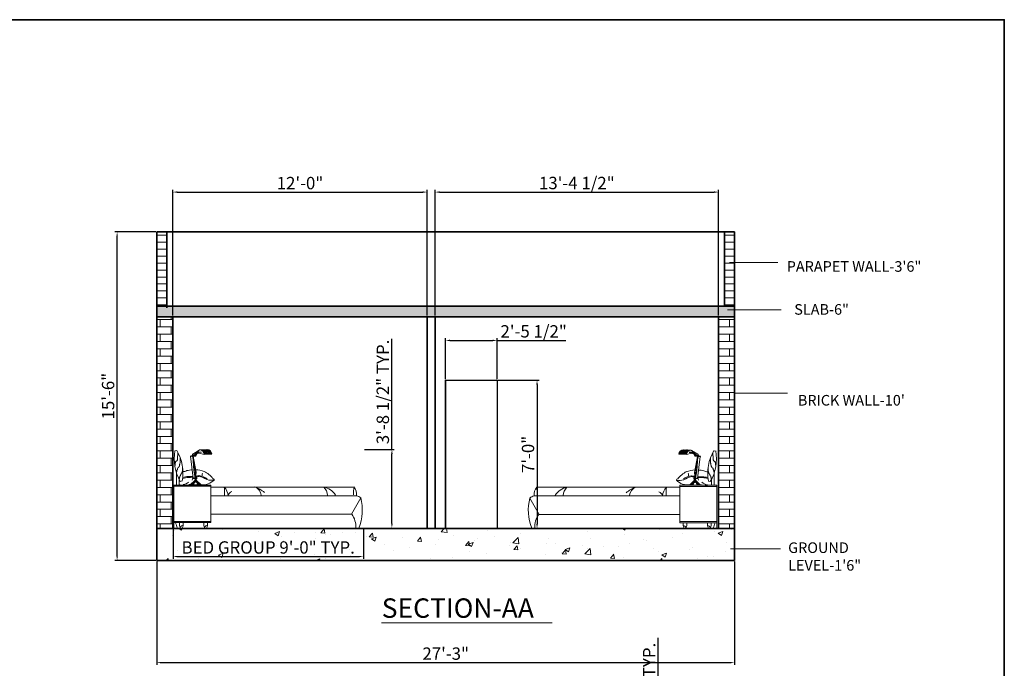
# Model space of a CAD drawing. Units: inches. Extents: x 1863 to 2938, y 1238 to 2492.
# Tile 12 of 12: x 2381 to 2938, y 2125 to 2492. Entities that reach past the tile are written whole.
import ezdxf

# ---------------------------------------------------------------- set-up
doc = ezdxf.new("R2010")
doc.units = ezdxf.units.IN
for name, color, linetype, lineweight in [('A-ANNO-DIMS', 2, 'Continuous', 18), ('A-ANNO-TEXT', 7, 'Continuous', 18), ('A-ANNO-TTLB', 7, 'Continuous', 35), ('A-DOOR', 3, 'Continuous', 25), ('A-FURN', 8, 'Continuous', 18), ('A-SECT', 7, 'Continuous', 35), ('A-SECT-PATT', 8, 'Continuous', 13), ('A-WALL-PATT', 8, 'Continuous', 13)]:
    doc.layers.add(name, color=color, linetype=linetype, lineweight=lineweight)
doc.styles.get("Standard").update_dxf_attribs({"font": 'arial.ttf'})
doc.dimstyles.new('ISO-25', dxfattribs={"dimtxt": 7, "dimasz": 2.5, "dimexe": 1.25, "dimexo": 0.625, "dimtad": 1, "dimdec": 0, "dimlunit": 3, "dimtxsty": 'Standard', "dimcen": 2.5, "dimadec": 0, "dimazin": 0, "dimtfac": 1, "dimtdec": 0, "dimtmove": 0, "dimatfit": 3, "dimfxl": 1, "dimarcsym": 0})

# ---------------------------------------------------------------- blocks, each defined once
blk = doc.blocks.new('A$C244A68C2')
for p, q in [((12, 836), (32, 839)), ((38, 746), (39, 750)), ((38, 739), (38, 746)), ((39, 750), (40, 756)), ((40, 759), (41, 762)), ((40, 756), (40, 759)), ((41, 782), (42, 783)), ((41, 779), (41, 782)), ((41, 775), (41, 779)), ((41, 762), (41, 775)), ((42, 786), (43, 787)), ((42, 783), (42, 786)), ((43, 790), (44, 791)), ((43, 787), (43, 790)), ((44, 791), (44, 812)), ((44, 812), (45, 812)), ((45, 812), (45, 814)), ((67, 766), (67, 705)), ((180, 780), (179, 780)), ((179, 778), (208, 538)), ((179, 778), (180, 777)), ((180, 779), (195, 781)), ((180, 779), (195, 780)), ((180, 778), (195, 777)), ((180, 778), (195, 778)), ((180, 778), (195, 777)), ((180, 777), (208, 539)), ((211, 788), (198, 785)), ((199, 781), (202, 778)), ((201, 778), (199, 781)), ((199, 781), (199, 781)), ((202, 778), (201, 778)), ((201, 774), (209, 776)), ((203, 799), (202, 786)), ((203, 799), (202, 786)), ((205, 801), (203, 801)), ((203, 799), (203, 786)), ((203, 799), (204, 799)), ((204, 799), (205, 787)), ((204, 799), (206, 787)), ((205, 800), (273, 843)), ((205, 801), (275, 843)), ((205, 775), (221, 621)), ((205, 775), (218, 623)), ((208, 782), (260, 825)), ((208, 779), (259, 822)), ((208, 778), (259, 821)), ((239, 779), (208, 779)), ((209, 777), (240, 605)), ((209, 776), (236, 608)), ((214, 783), (238, 783)), ((234, 779), (259, 822)), ((239, 779), (259, 822)), ((299, 822), (259, 822)), ((299, 821), (259, 821)), ((260, 814), (259, 814)), ((264, 816), (268, 815)), ((268, 815), (264, 816)), ((264, 816), (264, 816)), ((268, 815), (268, 815)), ((268, 810), (273, 811)), ((328, 797), (273, 811)), ((278, 845), (361, 850)), ((410, 801), (328, 797)), ((11, 670), (12, 676)), ((11, 670), (11, 670)), ((12, 676), (13, 681)), ((13, 681), (15, 686)), ((15, 695), (16, 699)), ((15, 686), (15, 695)), ((16, 707), (17, 708)), ((16, 699), (16, 707)), ((17, 712), (18, 715)), ((17, 708), (17, 712)), ((18, 716), (19, 719)), ((18, 715), (18, 716)), ((19, 719), (20, 719)), ((20, 719), (23, 722)), ((23, 722), (27, 723)), ((27, 724), (30, 725)), ((27, 723), (27, 724)), ((30, 725), (31, 728)), ((31, 728), (32, 729)), ((32, 729), (36, 732)), ((36, 732), (37, 735)), ((37, 736), (38, 739)), ((37, 735), (37, 736)), ((40, 640), (39, 637)), ((41, 644), (40, 640)), ((42, 650), (41, 646)), ((41, 646), (41, 645)), ((41, 645), (41, 644)), ((43, 651), (42, 650)), ((44, 652), (43, 652)), ((43, 652), (43, 651)), ((45, 652), (44, 652)), ((46, 653), (45, 652)), ((47, 654), (46, 653)), ((48, 655), (47, 654)), ((49, 655), (48, 655)), ((50, 656), (49, 655)), ((51, 657), (50, 656)), ((52, 657), (51, 657)), ((53, 658), (52, 658)), ((52, 658), (52, 657)), ((54, 659), (53, 658)), ((55, 662), (54, 659)), ((57, 663), (55, 662)), ((58, 665), (57, 665)), ((57, 665), (57, 663)), ((59, 667), (58, 666)), ((58, 666), (58, 665)), ((60, 671), (59, 668)), ((59, 668), (59, 667)), ((61, 675), (60, 672)), ((60, 672), (60, 671)), ((62, 679), (61, 676)), ((61, 676), (61, 675)), ((63, 683), (62, 682)), ((62, 682), (62, 679)), ((64, 692), (63, 688)), ((63, 688), (63, 683)), ((66, 699), (64, 692)), ((67, 705), (66, 699)), ((92, 616), (92, 640)), ((92, 640), (93, 640)), ((93, 640), (93, 659)), ((27, 602), (27, 465)), ((30, 603), (29, 602)), ((29, 602), (29, 598)), ((29, 598), (29, 598)), ((31, 611), (30, 610)), ((30, 610), (30, 603)), ((32, 614), (31, 613)), ((31, 613), (31, 611)), ((33, 619), (32, 618)), ((32, 618), (32, 614)), ((34, 624), (33, 620)), ((33, 620), (33, 619)), ((35, 627), (34, 626)), ((34, 626), (34, 624)), ((36, 628), (35, 627)), ((37, 631), (36, 630)), ((36, 630), (36, 628)), ((38, 634), (37, 631)), ((39, 637), (38, 636)), ((38, 636), (38, 634)), ((59, 526), (59, 536)), ((59, 536), (60, 536)), ((60, 536), (60, 543)), ((60, 543), (61, 543)), ((61, 543), (61, 544)), ((61, 544), (62, 544)), ((62, 544), (62, 549)), ((62, 549), (63, 549)), ((63, 549), (63, 552)), ((63, 552), (64, 552)), ((64, 552), (64, 556)), ((64, 556), (65, 556)), ((65, 559), (65, 561)), ((65, 561), (66, 561)), ((65, 556), (65, 559)), ((65, 559), (65, 559)), ((66, 561), (66, 562)), ((66, 562), (67, 562)), ((67, 562), (67, 564)), ((67, 564), (68, 564)), ((68, 564), (69, 564)), ((69, 565), (70, 566)), ((69, 564), (69, 565)), ((70, 566), (71, 567)), ((71, 567), (72, 571)), ((72, 572), (73, 573)), ((72, 571), (72, 572)), ((73, 574), (74, 575)), ((73, 573), (73, 574)), ((74, 575), (74, 577)), ((74, 577), (75, 577)), ((75, 579), (76, 580)), ((75, 577), (75, 579)), ((76, 580), (76, 582)), ((76, 582), (77, 582)), ((77, 583), (78, 584)), ((77, 582), (77, 583)), ((78, 588), (79, 589)), ((78, 587), (78, 588)), ((78, 586), (78, 587)), ((78, 584), (78, 586)), ((79, 589), (80, 589)), ((80, 589), (81, 590)), ((81, 590), (82, 591)), ((82, 591), (83, 591)), ((83, 591), (83, 592)), ((83, 592), (84, 592)), ((84, 592), (85, 593)), ((85, 594), (86, 595)), ((85, 593), (85, 594)), ((86, 595), (87, 599)), ((87, 599), (88, 600)), ((88, 600), (88, 604)), ((88, 604), (89, 604)), ((89, 604), (89, 606)), ((89, 606), (90, 606)), ((90, 606), (90, 608)), ((90, 608), (91, 608)), ((91, 612), (92, 613)), ((91, 608), (91, 612)), ((92, 615), (92, 616)), ((92, 613), (92, 615)), ((210, 539), (208, 539)), ((209, 538), (209, 538)), ((209, 537), (227, 536)), ((209, 537), (227, 536)), ((209, 537), (210, 537)), ((210, 538), (228, 540)), ((210, 538), (228, 540)), ((210, 537), (227, 537)), ((218, 623), (230, 541)), ((221, 621), (230, 541)), ((230, 536), (234, 535)), ((233, 534), (230, 536)), ((230, 536), (230, 536)), ((245, 544), (231, 542)), ((234, 535), (233, 534)), ((236, 608), (234, 542)), ((240, 605), (234, 543)), ((234, 564), (237, 564)), ((234, 564), (238, 564)), ((237, 564), (234, 564)), ((234, 561), (238, 562)), ((234, 561), (237, 562)), ((235, 561), (234, 542)), ((235, 563), (238, 564)), ((236, 561), (235, 542)), ((235, 561), (235, 542)), ((237, 561), (238, 543)), ((237, 561), (238, 543)), ((0, 0), (0, 465)), ((0, 465), (400, 465)), ((0, 453), (400, 453)), ((57, 529), (57, 465)), ((90, 509), (70, 505)), ((232, 519), (176, 467)), ((176, 467), (296, 467)), ((176, 466), (176, 465)), ((176, 465), (297, 465)), ((232, 519), (232, 529)), ((232, 519), (242, 519)), ((233, 529), (247, 532)), ((233, 519), (233, 530)), ((233, 519), (233, 529)), ((234, 519), (234, 530)), ((236, 519), (236, 530)), ((241, 519), (241, 531)), ((242, 519), (242, 531)), ((242, 519), (242, 531)), ((296, 467), (242, 519)), ((297, 465), (297, 466)), ((400, 465), (400, 60)), ((400, 444), (1950, 444)), ((400, 349), (1978, 349)), ((2023, 327), (1924, 150)), ((1924, 150), (400, 150)), ((400, 72), (0, 72)), ((400, 60), (0, 60)), ((2000, 0), (0, 0)), ((69, 0), (39, 0)), ((1970, 0), (2000, 0))]:
    blk.add_line(p, q)
for centre in [(200, 780), (266, 815)]:
    blk.add_circle(centre, 5.65)
for centre, radius, start, end in [((490, 750), 486, 169.7597, 210.2403), ((-388, 595), 486, 349.7597, 30.2403), ((179, 778), 1.33, 113.0446, 219.3657), ((179, 778), 0.665, 242.9995, 272.6955), ((179, 779), 0.499, 23.7236, 96.4275), ((178, 779), 1.65, 302.8629, 16.2974), ((178, 779), 0.993, 300.7534, 34.996), ((179, 779), 1.41, 300.6413, 40.8102), ((204, 800), 1.41, 113.0446, 219.3657), ((202, 800), 1.74, 302.8629, 16.2974), ((203, 800), 0.527, 23.7236, 96.4275), ((202, 800), 1.05, 300.7534, 34.996), ((203, 799), 0.701, 242.9995, 272.6955), ((203, 800), 1.49, 302.2124, 40.8102), ((212, 780), 4.54, 146.492, 201.5266), ((206, 786), 10.1, 287.8935, 311.557), ((208, 782), 6.25, 5.1761, 68.5727), ((222, 781), 2.75, 324.8716, 43.8406), ((223, 781), 2.75, 324.8716, 43.8406), ((289, 817), 30.1, 110.5321, 185.4329), ((278, 795), 50.1, 2.0446, 89.1762), ((285, 795), 50.1, 2.62, 89.1762), ((292, 797), 50.1, 0.9228, 81.157), ((309, 797), 50.1, 2.0096, 97.716), ((300, 797), 50.1, 1.4059, 83.743), ((317, 797), 50.1, 2.0154, 97.6411), ((326, 798), 50.1, 2.0212, 97.5649), ((335, 798), 50.1, 2.0446, 89.8396), ((344, 798), 50.1, 2.6306, 89.1762), ((352, 800), 50.1, 1.5315, 84.5393), ((360, 800), 50.1, 2.0446, 89.1762), ((188, 153), 396, 94.4237, 103.6768), ((188, 153), 406, 94.4237, 103.1785), ((102, 690), 79.6, 266.5082, 300.0492), ((220, 319), 312, 94.2751, 104.4301), ((161, 1136), 579, 269.5712, 274.3558), ((161, 1136), 588, 269.5712, 274.3996), ((247, 517), 49.6, 143.8256, 177.3514), ((208, 538), 0.549, 47.8474, 120.5513), ((209, 538), 1.47, 137.1685, 243.4896), ((208, 538), 1.09, 324.8773, 59.1199), ((207, 538), 1.82, 326.9868, 40.4213), ((209, 537), 0.731, 267.1233, 296.8194), ((209, 538), 1.46, 324.571, 61.0928), ((225, 543), 7.93, 47.5431, 107.8683), ((225, 542), 8.22, 45.6214, 105.6239), ((233, 536), 6.38, 116.914, 258.5276), ((233, 535), 5.43, 117.012, 254.6625), ((231, 538), 3.62, 54.3229, 113.5884), ((231, 537), 3.42, 88.4984, 107.6275), ((228, 535), 5.38, 317.0855, 61.4366), ((234, 562), 1.61, 113.0446, 254.6581), ((234, 563), 0.913, 50.4535, 109.7189), ((234, 563), 0.864, 84.629, 103.758), ((234, 562), 1.37, 113.1426, 250.793), ((233, 562), 1.64, 295.9717, 55.8772), ((233, 562), 1.1, 315.8031, 60.4731), ((234, 562), 0.947, 260.6456, 290.3416), ((230, 535), 6.5, 299.8411, 59.7467), ((220, 319), 312, 69.9385, 87.115), ((237, 563), 1.64, 301.136, 71.7859), ((161, 1136), 579, 277.6123, 280.9344), ((161, 1136), 588, 277.4426, 280.9344), ((243, 538), 6.48, 305.0055, 75.6553), ((224, 315), 248, 57.6744, 78.9535), ((224, 315), 258, 57.6744, 78.9535), ((336, 576), 31.1, 141.8486, 203.2325), ((219, 384), 253, 36.2927, 64.7019), ((422, 521), 13.7, 351.6123, 92.6357), ((116, 662), 200, 252.6794, 279.5672), ((84, 593), 124, 277.542, 309.9334), ((258, 63), 417, 100.9046, 105.0614), ((176, 466), 0.81, 90, 180), ((232, 533), 3.75, 264.5151, 294.2111), ((311, 645), 177, 264.2572, 314.636), ((296, 466), 0.81, 360, 90), ((405, 650), 134, 250.0666, 283.0972), ((-655, 373), 1203, 358.8801, 3.375), ((439, 340), 148, 3.5443, 44.2346), ((834, 341), 112, 7.9131, 67.3602), ((739, 84), 386, 51.1586, 69.1463), ((1526, 348), 136, 1.9043, 44.8247), ((1591, 263), 183, 30.3408, 80.0939), ((2269, 374), 326, 167.6533, 182.7628), ((1855, 364), 124, 353.2313, 40.2408), ((648, 336), 61.5, 109.2631, 167.6798), ((1967, 270), 80, 45, 81.6372), ((1523, 198), 517, 337.4954, 14.4201), ((1736, 10), 235, 357.5091, 36.5889), ((514, 197), 514, 195.5801, 202.5597), ((158, 45), 98.5, 171.4719, 207.4528), ((107, -17), 46.6, 97.2386, 147.0434), ((301, 10), 232, 181.8198, 182.4988), ((4, 45), 98.5, 332.5472, 8.5281), ((422, 45), 98.5, 171.4719, 207.4528), ((370, -17), 46.6, 97.2386, 147.0434), ((267, 45), 98.5, 332.5472, 8.5281)]:
    blk.add_arc(centre, radius, start, end)
for points in [[(200, 774), (201, 774), (201, 775), (202, 775), (202, 775), (203, 776), (203, 777), (204, 778), (204, 779), (204, 781), (204, 781), (203, 782), (203, 783), (202, 784), (202, 784), (201, 784), (201, 784), (200, 784), (200, 784), (200, 784), (200, 784)], [(266, 810), (267, 810), (267, 810), (268, 811), (268, 811), (269, 812), (269, 813), (270, 814), (270, 815), (270, 817), (269, 817), (269, 818), (268, 819), (268, 820), (267, 820), (266, 820), (266, 820), (266, 820), (266, 820), (266, 820), (266, 820)], [(231, 530), (232, 530), (232, 530), (233, 531), (234, 531), (234, 532), (235, 533), (235, 534), (235, 535), (235, 537), (235, 537), (234, 538), (234, 539), (233, 540), (233, 540), (232, 540), (232, 540), (231, 540), (231, 540), (231, 540), (231, 540)], [(234, 561), (234, 561), (234, 561), (234, 561), (234, 561), (234, 562), (234, 562), (235, 562), (235, 562), (235, 563), (235, 563), (234, 563), (234, 563), (234, 563), (234, 564), (234, 564), (234, 564), (234, 564), (234, 564), (234, 564), (234, 564)]]:
    blk.add_open_spline(points, degree=3, knots=[3.294068, 3.294068, 3.294068, 3.294068, 3.647859, 3.647859, 4.043866, 4.043866, 4.439873, 4.439873, 4.83588, 4.83588, 5.231886, 5.231886, 5.627893, 5.627893, 6.0239, 6.0239, 6.283185, 6.283185, 6.283185, 6.295262, 6.295262, 6.295262, 6.295262])
for p in [(202, 786), (202, 785), (203, 786), (203, 785), (204, 786), (204, 786), (204, 785), (204, 784), (205, 786), (205, 786), (205, 785), (205, 784), (205, 783), (205, 776), (205, 775), (205, 775), (205, 775), (206, 786), (206, 786), (206, 785), (206, 777), (206, 776), (206, 776), (206, 776), (207, 786), (207, 783), (208, 787), (208, 786), (208, 786), (208, 785), (208, 777), (208, 777), (208, 777), (209, 787), (209, 787), (209, 787), (209, 786), (209, 785), (209, 784), (209, 784), (209, 777), (209, 777), (210, 787), (210, 787), (210, 787), (210, 787), (210, 786), (210, 778), (210, 777), (211, 787), (211, 786), (211, 778), (211, 777), (212, 787), (212, 786), (212, 786), (212, 784), (213, 785), (234, 542), (234, 541), (234, 541), (235, 542), (235, 541), (235, 541), (235, 540), (236, 542), (236, 541), (236, 541), (236, 541), (236, 540), (236, 540), (237, 543), (237, 542), (237, 542), (237, 541), (237, 541), (237, 541), (237, 540), (238, 543), (238, 542), (238, 542), (238, 542), (238, 540), (238, 538), (239, 542), (239, 541), (239, 541), (239, 539), (240, 543), (240, 541), (240, 541), (241, 543), (241, 543), (241, 542), (242, 543), (242, 543), (242, 542), (242, 542), (242, 540), (243, 543), (243, 543), (243, 543), (244, 544), (244, 543), (244, 542), (244, 540), (244, 540), (245, 544), (245, 544), (245, 544), (245, 543), (245, 533), (245, 533), (245, 533), (246, 543), (246, 543), (246, 542), (246, 534), (246, 533), (247, 543), (247, 543), (247, 541), (247, 535), (247, 534), (247, 534), (248, 541), (248, 537), (248, 536), (248, 535), (248, 535), (248, 535), (248, 535), (248, 534), (181, 468), (182, 469), (183, 470), (185, 472), (185, 471), (186, 470), (186, 470), (186, 468), (186, 468), (186, 467), (187, 473), (188, 474), (188, 473), (188, 471), (188, 471), (188, 470), (189, 473), (190, 474), (190, 474), (190, 470), (190, 470), (191, 478), (191, 474), (191, 471), (193, 474), (193, 474), (193, 473), (193, 469), (194, 478), (194, 473), (194, 471), (195, 476), (195, 473), (195, 471), (196, 477), (197, 480), (197, 473), (197, 469), (198, 470), (198, 469), (198, 469), (199, 482), (201, 482), (201, 470), (202, 486), (202, 482), (202, 469), (204, 484), (205, 481), (206, 485), (206, 477), (206, 469), (206, 468), (207, 491), (207, 489), (207, 487), (207, 474), (207, 473), (208, 487), (208, 482), (209, 491), (210, 491), (210, 489), (210, 484), (210, 472), (211, 496), (211, 470), (211, 470), (212, 493), (212, 485), (212, 475), (214, 498), (214, 487), (215, 500), (215, 499), (215, 476), (216, 500), (216, 498), (216, 497), (216, 489), (216, 489), (216, 484), (216, 480), (217, 502), (217, 499), (218, 504), (219, 504), (219, 503), (219, 502), (219, 501), (219, 483), (220, 506), (220, 505), (221, 504), (221, 504), (221, 498), (221, 492), (222, 506), (222, 506), (222, 494), (223, 508), (223, 501), (223, 498), (224, 508), (224, 506), (224, 506), (224, 504), (225, 510), (225, 508), (225, 498), (226, 511), (226, 509), (226, 503), (227, 513), (227, 511), (227, 507), (227, 504), (228, 514), (228, 511), (228, 508), (229, 512), (229, 512), (229, 511), (229, 508), (229, 507), (230, 513), (230, 512), (230, 511), (230, 503), (231, 516), (231, 515), (231, 514), (231, 507), (232, 516), (233, 517), (233, 514), (233, 512), (233, 510), (234, 517), (234, 513), (234, 512), (235, 519), (235, 517), (235, 517), (235, 516), (235, 515), (235, 514), (235, 512), (236, 532), (236, 517), (236, 517), (236, 497), (237, 532), (237, 532), (237, 504), (237, 500), (238, 532), (238, 515), (238, 512), (238, 497), (239, 532), (239, 532), (239, 508), (240, 532), (241, 533), (241, 533), (243, 533), (243, 532), (243, 513), (243, 512), (243, 506), (244, 514), (244, 512), (244, 511), (244, 508), (245, 513), (245, 511), (245, 511), (246, 511), (246, 506), (246, 502), (246, 500), (247, 510), (247, 509), (248, 508), (248, 495), (249, 508), (249, 506), (249, 506), (249, 504), (249, 502), (250, 508), (250, 506), (251, 506), (251, 504), (251, 498), (251, 492), (252, 506), (252, 505), (252, 504), (253, 467), (254, 504), (254, 503), (254, 502), (254, 501), (254, 483), (254, 473), (255, 504), (255, 499), (255, 495), (255, 493), (255, 486), (255, 484), (256, 502), (256, 500), (256, 498), (256, 497), (257, 500), (257, 499), (258, 498), (258, 487), (258, 478), (258, 471), (259, 498), (259, 495), (259, 491), (260, 494), (260, 493), (260, 490), (260, 479), (260, 472), (260, 467), (261, 496), (261, 489), (261, 485), (262, 488), (262, 487), (262, 484), (263, 491), (263, 489), (263, 484), (264, 491), (264, 481), (264, 471), (264, 471), (265, 491), (265, 489), (265, 487), (265, 487), (265, 482), (266, 485), (266, 484), (266, 470), (266, 467), (267, 478), (267, 469), (267, 469), (267, 467), (268, 481), (269, 484), (269, 482), (269, 481), (269, 473), (270, 486), (270, 482), (270, 477), (270, 469), (271, 488), (271, 482), (271, 470), (273, 476), (273, 470), (274, 482), (274, 469), (276, 480), (277, 480), (280, 471), (280, 469), (281, 474), (281, 471), (282, 475), (282, 470), (284, 471), (285, 473), (285, 470), (287, 470), (288, 470), (288, 469), (290, 469), (291, 467)]:
    blk.add_point(p)
blk = doc.blocks.new('*D38')
at = {"layer": 'A-ANNO-DIMS', "color": 0, "lineweight": -2, "transparency": 16777216}
for p, q in [((2467.74, 2203.68), (2467.74, 2186.89)), ((2575.51, 2203.68), (2575.51, 2186.89)), ((2470.24, 2188.14), (2573.01, 2188.14))]:
    blk.add_line(p, q, dxfattribs=at)
at = {"layer": 'A-ANNO-DIMS', "color": 0, "transparency": 16777216}
for points in [[(2470.24, 2188.55), (2470.24, 2187.72), (2467.74, 2188.14)], [(2573.01, 2188.55), (2573.01, 2187.72), (2575.51, 2188.14)]]:
    blk.add_solid(points, dxfattribs=at)
at = {"layer": 'Defpoints', "color": 0, "transparency": 16777216}
for p in [(2467.74, 2204.3), (2575.51, 2204.3), (2575.51, 2188.14)]:
    blk.add_point(p, dxfattribs=at)
at = {"layer": 'A-ANNO-DIMS', "color": 0, "transparency": 16777216, "insert": (2521.62, 2192.38), "char_height": 7, "attachment_point": 5}
blk.add_mtext('BED GROUP 9\'-0" TYP.', dxfattribs=at)
blk = doc.blocks.new('*D39')
at = {"layer": 'A-ANNO-DIMS', "color": 0, "lineweight": -2, "transparency": 16777216}
for p, q in [((2591.67, 2248.76), (2591.67, 2311.48)), ((2576.13, 2248.76), (2592.92, 2248.76)), ((2591.67, 2206.8), (2591.67, 2246.26)), ((2576.13, 2204.3), (2592.92, 2204.3))]:
    blk.add_line(p, q, dxfattribs=at)
at = {"layer": 'A-ANNO-DIMS', "color": 0, "transparency": 16777216}
for points in [[(2591.26, 2246.26), (2592.09, 2246.26), (2591.67, 2248.76)], [(2591.26, 2206.8), (2592.09, 2206.8), (2591.67, 2204.3)]]:
    blk.add_solid(points, dxfattribs=at)
at = {"layer": 'Defpoints', "color": 0, "transparency": 16777216}
for p in [(2575.51, 2248.76), (2591.67, 2248.76), (2575.51, 2204.3)]:
    blk.add_point(p, dxfattribs=at)
at = {"layer": 'A-ANNO-DIMS', "color": 0, "transparency": 16777216, "insert": (2587.43, 2281.37), "char_height": 7, "attachment_point": 5, "rotation": 90}
blk.add_mtext('3\'-8 1/2" TYP.', dxfattribs=at)
blk = doc.blocks.new('*D44')
at = {"layer": 'A-ANNO-DIMS', "color": 0, "lineweight": -2, "transparency": 16777216}
for p, q in [((2742.49, 2018.92), (2742.49, 2142.19)), ((2739.01, 2018.92), (2743.74, 2018.92)), ((2742.49, 1994.04), (2742.49, 2016.42)), ((2739.01, 1991.54), (2743.74, 1991.54))]:
    blk.add_line(p, q, dxfattribs=at)
at = {"layer": 'A-ANNO-DIMS', "color": 0, "transparency": 16777216}
for points in [[(2742.07, 2016.42), (2742.91, 2016.42), (2742.49, 2018.92)], [(2742.07, 1994.04), (2742.91, 1994.04), (2742.49, 1991.54)]]:
    blk.add_solid(points, dxfattribs=at)
at = {"layer": 'Defpoints', "color": 0, "transparency": 16777216}
for p in [(2738.38, 2018.92), (2742.49, 2018.92), (2738.38, 1991.54)]:
    blk.add_point(p, dxfattribs=at)
at = {"layer": 'A-ANNO-DIMS', "color": 0, "transparency": 16777216, "insert": (2738.24, 2081.8), "char_height": 7, "attachment_point": 5, "rotation": 90}
blk.add_mtext('BATH DOOR 2\'-3 1/2" TYP.', dxfattribs=at)
blk = doc.blocks.new('*D87')
at = {"layer": 'A-ANNO-DIMS', "color": 0, "lineweight": -2, "transparency": 16777216}
for p, q in [((2458.63, 2185.37), (2458.63, 2126.81)), ((2785.63, 2185.37), (2785.63, 2126.81)), ((2461.13, 2128.06), (2783.13, 2128.06))]:
    blk.add_line(p, q, dxfattribs=at)
at = {"layer": 'A-ANNO-DIMS', "color": 0, "transparency": 16777216}
for points in [[(2461.13, 2128.47), (2461.13, 2127.64), (2458.63, 2128.06)], [(2783.13, 2128.47), (2783.13, 2127.64), (2785.63, 2128.06)]]:
    blk.add_solid(points, dxfattribs=at)
at = {"layer": 'Defpoints', "color": 0, "transparency": 16777216}
for p in [(2458.63, 2185.99), (2785.63, 2185.99), (2785.63, 2128.06)]:
    blk.add_point(p, dxfattribs=at)
at = {"layer": 'A-ANNO-DIMS', "color": 0, "transparency": 16777216, "insert": (2622.13, 2132.26), "char_height": 7, "attachment_point": 5}
blk.add_mtext('27\'-3"', dxfattribs=at)
blk = doc.blocks.new('*D88')
at = {"layer": 'A-ANNO-DIMS', "color": 0, "lineweight": -2, "transparency": 16777216}
for p, q in [((2458.01, 2371.99), (2434.83, 2371.99)), ((2436.08, 2188.49), (2436.08, 2369.49)), ((2458.01, 2185.99), (2434.83, 2185.99))]:
    blk.add_line(p, q, dxfattribs=at)
at = {"layer": 'A-ANNO-DIMS', "color": 0, "transparency": 16777216}
for points in [[(2435.66, 2369.49), (2436.5, 2369.49), (2436.08, 2371.99)], [(2435.66, 2188.49), (2436.5, 2188.49), (2436.08, 2185.99)]]:
    blk.add_solid(points, dxfattribs=at)
at = {"layer": 'Defpoints', "color": 0, "transparency": 16777216}
for p in [(2436.08, 2371.99), (2458.63, 2371.99), (2458.63, 2185.99)]:
    blk.add_point(p, dxfattribs=at)
at = {"layer": 'A-ANNO-DIMS', "color": 0, "transparency": 16777216, "insert": (2431.88, 2278.99), "char_height": 7, "attachment_point": 5, "rotation": 90}
blk.add_mtext('15\'-6"', dxfattribs=at)
blk = doc.blocks.new('*D89')
at = {"layer": 'A-ANNO-DIMS', "color": 0, "lineweight": -2, "transparency": 16777216}
for p, q in [((2467.63, 2324.62), (2467.63, 2395.79)), ((2470.13, 2394.54), (2609.13, 2394.54)), ((2611.63, 2324.62), (2611.63, 2395.79))]:
    blk.add_line(p, q, dxfattribs=at)
at = {"layer": 'A-ANNO-DIMS', "color": 0, "transparency": 16777216}
for points in [[(2470.13, 2394.96), (2470.13, 2394.12), (2467.63, 2394.54)], [(2609.13, 2394.96), (2609.13, 2394.12), (2611.63, 2394.54)]]:
    blk.add_solid(points, dxfattribs=at)
at = {"layer": 'Defpoints', "color": 0, "transparency": 16777216}
for p in [(2611.63, 2394.54), (2467.63, 2323.99), (2611.63, 2323.99)]:
    blk.add_point(p, dxfattribs=at)
at = {"layer": 'A-ANNO-DIMS', "color": 0, "transparency": 16777216, "insert": (2539.63, 2398.74), "char_height": 7, "attachment_point": 5}
blk.add_mtext('12\'-0"', dxfattribs=at)
blk = doc.blocks.new('*D90')
at = {"layer": 'A-ANNO-DIMS', "color": 0, "lineweight": -2, "transparency": 16777216}
for p, q in [((2616.13, 2324.62), (2616.13, 2395.79)), ((2618.63, 2394.54), (2774.13, 2394.54)), ((2776.63, 2324.62), (2776.63, 2395.79))]:
    blk.add_line(p, q, dxfattribs=at)
at = {"layer": 'A-ANNO-DIMS', "color": 0, "transparency": 16777216}
for points in [[(2618.63, 2394.96), (2618.63, 2394.12), (2616.13, 2394.54)], [(2774.13, 2394.96), (2774.13, 2394.12), (2776.63, 2394.54)]]:
    blk.add_solid(points, dxfattribs=at)
at = {"layer": 'Defpoints', "color": 0, "transparency": 16777216}
for p in [(2776.63, 2394.54), (2616.13, 2323.99), (2776.63, 2323.99)]:
    blk.add_point(p, dxfattribs=at)
at = {"layer": 'A-ANNO-DIMS', "color": 0, "transparency": 16777216, "insert": (2696.38, 2398.79), "char_height": 7, "attachment_point": 5}
blk.add_mtext('13\'-4 1/2"', dxfattribs=at)
blk = doc.blocks.new('*D91')
at = {"layer": 'A-ANNO-DIMS', "color": 0, "lineweight": -2, "transparency": 16777216}
for p, q in [((2651.91, 2287.99), (2675.09, 2287.99)), ((2673.84, 2285.49), (2673.84, 2206.49)), ((2651.91, 2203.99), (2675.09, 2203.99))]:
    blk.add_line(p, q, dxfattribs=at)
at = {"layer": 'A-ANNO-DIMS', "color": 0, "transparency": 16777216}
for points in [[(2673.42, 2285.49), (2674.25, 2285.49), (2673.84, 2287.99)], [(2673.42, 2206.49), (2674.25, 2206.49), (2673.84, 2203.99)]]:
    blk.add_solid(points, dxfattribs=at)
at = {"layer": 'Defpoints', "color": 0, "transparency": 16777216}
for p in [(2651.29, 2287.99), (2651.29, 2203.99), (2673.84, 2203.99)]:
    blk.add_point(p, dxfattribs=at)
at = {"layer": 'A-ANNO-DIMS', "color": 0, "transparency": 16777216, "insert": (2669.64, 2245.99), "char_height": 7, "attachment_point": 5, "rotation": 90}
blk.add_mtext('7\'-0"', dxfattribs=at)
blk = doc.blocks.new('*D92')
at = {"layer": 'A-ANNO-DIMS', "color": 0, "lineweight": -2, "transparency": 16777216}
for p, q in [((2622.04, 2288.62), (2622.04, 2311.79)), ((2624.54, 2310.54), (2648.79, 2310.54)), ((2651.29, 2288.62), (2651.29, 2311.79)), ((2651.29, 2310.54), (2690.08, 2310.54))]:
    blk.add_line(p, q, dxfattribs=at)
at = {"layer": 'A-ANNO-DIMS', "color": 0, "transparency": 16777216}
for points in [[(2624.54, 2310.96), (2624.54, 2310.12), (2622.04, 2310.54)], [(2648.79, 2310.96), (2648.79, 2310.12), (2651.29, 2310.54)]]:
    blk.add_solid(points, dxfattribs=at)
at = {"layer": 'Defpoints', "color": 0, "transparency": 16777216}
for p in [(2651.29, 2310.54), (2622.04, 2287.99), (2651.29, 2287.99)]:
    blk.add_point(p, dxfattribs=at)
at = {"layer": 'A-ANNO-DIMS', "color": 0, "transparency": 16777216, "insert": (2671.93, 2314.78), "char_height": 7, "attachment_point": 5}
blk.add_mtext('2\'-5 1/2"', dxfattribs=at)

msp = doc.modelspace()

# ---------------------------------------------------------------- hatches: boundary and pattern name
at = {"layer": 'A-SECT-PATT'}
h = msp.add_hatch(dxfattribs=at)
h.set_pattern_fill('AR-CONC', color=256, scale=0.045, style=0)
h.paths.add_polyline_path([(2458.63, 2323.99), (2785.63, 2323.99), (2785.63, 2329.99), (2458.63, 2329.99)])
h = msp.add_hatch(dxfattribs=at)
h.set_pattern_fill('AR-CONC', color=256, scale=0.15, style=0)
h.paths.add_polyline_path([(2458.63, 2185.99), (2785.63, 2185.99), (2785.63, 2203.99), (2458.63, 2203.99)])
at = {"layer": 'A-WALL-PATT'}
h = msp.add_hatch(dxfattribs=at)
h.set_pattern_fill('LINE', color=256, scale=1.24, style=0)
h.paths.add_polyline_path([(2458.63, 2329.99), (2464.19, 2329.99), (2464.19, 2371.99), (2458.63, 2371.99)])
h = msp.add_hatch(dxfattribs=at)
h.set_pattern_fill('LINE', color=256, scale=1.24, style=0)
h.paths.add_polyline_path([(2780.05, 2329.99), (2785.63, 2329.99), (2785.63, 2371.99), (2780.05, 2371.99)])
h = msp.add_hatch(dxfattribs=at)
h.set_pattern_fill('AR-BRSTD', color=256, scale=0.061, style=0)
h.paths.add_polyline_path([(2458.63, 2203.99), (2467.63, 2203.99), (2467.63, 2323.99), (2458.63, 2323.99)])
h = msp.add_hatch(dxfattribs=at)
h.set_pattern_fill('AR-BRSTD', color=256, scale=0.061, style=0)
h.paths.add_polyline_path([(2776.63, 2203.99), (2785.63, 2203.99), (2785.63, 2323.99), (2776.63, 2323.99)])

# ---------------------------------------------------------------- linework, layer by layer
at = {"layer": 'A-ANNO-TEXT'}
for p, q in [((2782.84, 2354.68), (2810.09, 2354.68)), ((2781.77, 2327.92), (2811.99, 2327.92)), ((2785.63, 2280.67), (2815.7, 2280.67)), ((2783.39, 2192.59), (2811.67, 2192.59)), ((2585.71, 2150.61), (2682.44, 2150.61))]:
    msp.add_line(p, q, dxfattribs=at)
at = {"layer": 'A-ANNO-TTLB'}
msp.add_lwpolyline([(1863.2, 2492.19), (2938.41, 2492.19), (2938.41, 1253.47), (1863.2, 1253.47)], close=True, dxfattribs=at)
at = {"layer": 'A-DOOR'}
for p, q in [((2622.04, 2287.99), (2622.04, 2203.99)), ((2622.04, 2203.99), (2622.04, 2287.99)), ((2622.04, 2287.99), (2651.29, 2287.99)), ((2651.29, 2287.99), (2651.29, 2203.99))]:
    msp.add_line(p, q, dxfattribs=at)
at = {"layer": 'A-SECT'}
for p, q in [((2458.63, 2371.99), (2458.63, 2185.99)), ((2458.63, 2371.99), (2785.63, 2371.99)), ((2464.19, 2329.05), (2464.19, 2371.99)), ((2780.05, 2329.99), (2780.05, 2371.99)), ((2785.63, 2371.99), (2785.63, 2185.99)), ((2458.63, 2329.99), (2785.63, 2329.99)), ((2458.63, 2323.99), (2785.63, 2323.99)), ((2467.63, 2323.99), (2467.63, 2203.99)), ((2611.63, 2323.99), (2611.63, 2203.99)), ((2616.13, 2323.99), (2616.13, 2203.99)), ((2776.63, 2323.99), (2776.63, 2203.99)), ((2458.63, 2203.99), (2785.63, 2203.99)), ((2458.63, 2185.99), (2785.63, 2185.99))]:
    msp.add_line(p, q, dxfattribs=at)

# ---------------------------------------------------------------- block references
at = {"layer": 'A-FURN', "yscale": 0.0523142138983917, "zscale": 0.0523142138983917}
for p, xscale in [((2468.2, 2204.3), 0.0523142138983917), ((2775.63, 2204.18), -0.0523142138983917)]:
    msp.add_blockref('A$C244A68C2', p, dxfattribs=dict(at, xscale=xscale))

# ---------------------------------------------------------------- texts
at = {"layer": 'A-ANNO-TEXT', "attachment_point": 1}
for s, width, insert, char_height in [('PARAPET WALL-3\'6"', 114.3843, (2815.22, 2355.43), 6), ('SLAB-6"', 81.9754, (2819.48, 2331.1), 6), ("BRICK WALL-10'", 211.4644, (2821.53, 2279.64), 6), ('GROUND LEVEL-1\'6"', 65.94, (2816.02, 2196.17), 6), ('SECTION-AA', 293.6592, (2585.9, 2164.45), 11)]:
    msp.add_mtext_dynamic_manual_height_columns(s, width=width, gutter_width=12.5, heights=[0], dxfattribs=dict(at, insert=insert, char_height=char_height))

# ---------------------------------------------------------------- dimensions: what is measured, and where the dimension line sits
at = {"layer": 'A-ANNO-DIMS'}
for base, p1, p2, picture, middle in [((2776.63, 2394.54), (2616.13, 2323.99), (2776.63, 2323.99), '*D90', (2696.38, 2398.79)), ((2611.63, 2394.54), (2467.63, 2323.99), (2611.63, 2323.99), '*D89', (2539.63, 2398.74)), ((2651.287, 2310.5403), (2622.0367, 2287.9903), (2651.287, 2287.9903), '*D92', (2671.9311, 2314.7847)), ((2785.63, 2128.06), (2458.63, 2185.99), (2785.63, 2185.99), '*D87', (2622.13, 2132.26))]:
    dim = msp.add_linear_dim(base=base, p1=p1, p2=p2, dimstyle='ISO-25', override={"dimdec": 1, "dimlfac": 1, "dimrnd": 0, "dimzin": 1, "dimdsep": 46, "dimlunit": 4, "dimfrac": 2}, dxfattribs=at)
    dim.commit()
    dim.dimension.update_dxf_attribs({"geometry": picture, "text_midpoint": middle})
for base, p1, p2, angle, picture, middle in [((2436.08, 2371.99), (2458.63, 2185.99), (2458.63, 2371.99), 90, '*D88', (2431.88, 2278.99)), ((2673.84, 2203.99), (2651.29, 2287.99), (2651.29, 2203.99), 270, '*D91', (2669.64, 2245.99))]:
    dim = msp.add_linear_dim(base=base, p1=p1, p2=p2, angle=angle, dimstyle='ISO-25', override={"dimdec": 1, "dimlfac": 1, "dimrnd": 0, "dimzin": 1, "dimdsep": 46, "dimlunit": 4, "dimfrac": 2}, dxfattribs=at)
    dim.commit()
    dim.dimension.update_dxf_attribs({"geometry": picture, "text_midpoint": middle})
for base, p1, p2, text, picture, middle in [((2591.67, 2248.76), (2575.51, 2204.3), (2575.51, 2248.76), '<> TYP.', '*D39', (2587.43, 2281.37)), ((2742.49, 2018.92), (2738.38, 1991.54), (2738.38, 2018.92), 'BATH DOOR <> TYP.', '*D44', (2738.24, 2081.8))]:
    dim = msp.add_linear_dim(base=base, p1=p1, p2=p2, angle=90, text=text, dimstyle='ISO-25', override={"dimdec": 1, "dimlfac": 1, "dimrnd": 0, "dimzin": 1, "dimdsep": 46, "dimlunit": 4, "dimfrac": 2}, dxfattribs=at)
    dim.commit()
    dim.dimension.update_dxf_attribs({"geometry": picture, "text_midpoint": middle})
dim = msp.add_linear_dim(base=(2575.51, 2188.14), p1=(2467.74, 2204.3), p2=(2575.51, 2204.3), text='BED GROUP <> TYP.', dimstyle='ISO-25', override={"dimdec": 1, "dimlfac": 1, "dimrnd": 0, "dimzin": 1, "dimdsep": 46, "dimlunit": 4, "dimfrac": 2}, dxfattribs=at)
dim.commit()
dim.dimension.update_dxf_attribs({"geometry": '*D38', "text_midpoint": (2521.62, 2192.38)})

doc.saveas('drawing.dxf')
